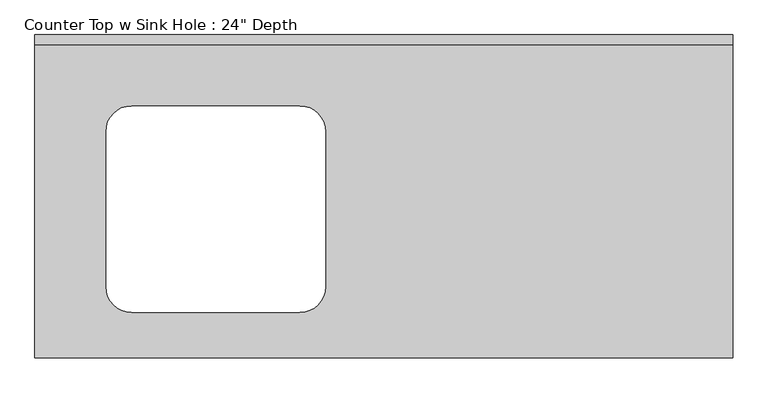
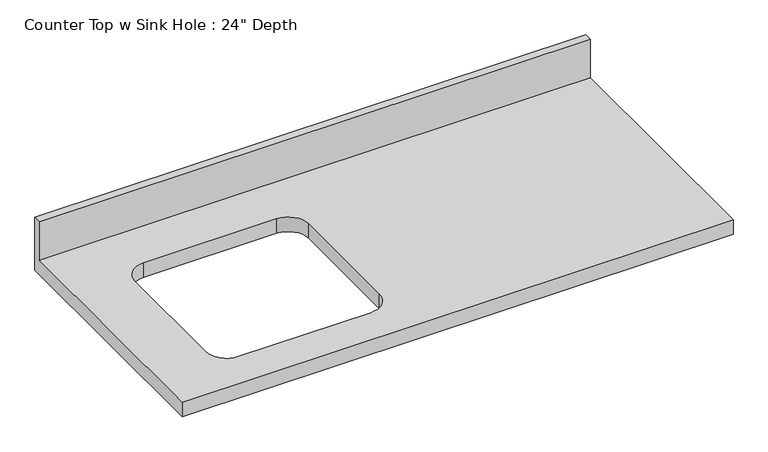
"""IFC4 building model written with IfcOpenShell, lengths in millimetres: furniture geometry."""

from ifc_helpers import new_model, si_unit, frame, origin, place, context, project, spatial, polyline, circle_curve, source, transform, mapped, element, save
from ifc_brep_helpers import plane_surface, revolved_surface, advanced_brep


def furniture_b3f308bd(model_context):
    return source(origin(), model_context, "Body", "AdvancedBrep", [
        advanced_brep(
        [(-1200.4622951, -635.0, 914.4), (171.1377049, -635.0, 914.4), (171.1377049, -19.05, 914.4), (-1200.4622951, -19.05, 914.4), (-1009.9622951, -139.7, 914.4), (-679.7622951, -139.7, 914.4), (-628.9622951, -190.5, 914.4), (-628.9622951, -495.3, 914.4), (-679.7622951, -546.1, 914.4), (-1009.9622951, -546.1, 914.4), (-1060.7622951, -495.3, 914.4), (-1060.7622951, -190.5, 914.4), (171.1377049, 0.0, 876.3), (171.1377049, -635.0, 876.3), (-1200.4622951, -635.0, 876.3), (-1200.4622951, 0.0, 876.3), (-679.7622951, -139.7, 876.3), (-1009.9622951, -139.7, 876.3), (-1060.7622951, -190.5, 876.3), (-1060.7622951, -495.3, 876.3), (-1009.9622951, -546.1, 876.3), (-679.7622951, -546.1, 876.3), (-628.9622951, -495.3, 876.3), (-628.9622951, -190.5, 876.3), (-1200.4622951, 0.0, 1016.0), (171.1377049, 0.0, 1016.0), (-1200.4622951, -19.05, 1016.0), (171.1377049, -19.05, 1016.0)],
        [
            (0, 1),
            (1, 2),
            (2, 3),
            (3, 0),
            (4, 5),
            (5, 6, circle_curve(frame((-679.7622951, -190.5, 914.4), z_axis=(0.0, 0.0, -1.0), x_axis=(1.0, 0.0, 0.0)), 50.8)),
            (6, 7),
            (7, 8, circle_curve(frame((-679.7622951, -495.3, 914.4), z_axis=(0.0, 0.0, -1.0), x_axis=(1.0, 0.0, 0.0)), 50.8)),
            (8, 9),
            (9, 10, circle_curve(frame((-1009.9622951, -495.3, 914.4), z_axis=(0.0, 0.0, -1.0), x_axis=(1.0, 0.0, 0.0)), 50.8)),
            (10, 11),
            (11, 4, circle_curve(frame((-1009.9622951, -190.5, 914.4), z_axis=(0.0, 0.0, -1.0), x_axis=(1.0, 0.0, 0.0)), 50.8)),
            (12, 13),
            (13, 14),
            (14, 15),
            (15, 12),
            (16, 17),
            (17, 18, circle_curve(frame((-1009.9622951, -190.5, 876.3), z_axis=(0.0, 0.0, 1.0), x_axis=(1.0, 0.0, 0.0)), 50.8)),
            (18, 19),
            (19, 20, circle_curve(frame((-1009.9622951, -495.3, 876.3), z_axis=(0.0, 0.0, 1.0), x_axis=(1.0, 0.0, 0.0)), 50.8)),
            (20, 21),
            (21, 22, circle_curve(frame((-679.7622951, -495.3, 876.3), z_axis=(0.0, 0.0, 1.0), x_axis=(1.0, 0.0, 0.0)), 50.8)),
            (22, 23),
            (23, 16, circle_curve(frame((-679.7622951, -190.5, 876.3), z_axis=(0.0, 0.0, 1.0), x_axis=(1.0, 0.0, 0.0)), 50.8)),
            (15, 24),
            (24, 25),
            (25, 12),
            (14, 0),
            (3, 26),
            (26, 24),
            (13, 1),
            (25, 27),
            (27, 2),
            (4, 17),
            (16, 5),
            (11, 18),
            (10, 19),
            (9, 20),
            (8, 21),
            (7, 22),
            (6, 23),
            (26, 27),
        ],
        [
            plane_surface(frame((-1200.4622951, 0.0, 914.4), z_axis=(0.0, 0.0, 1.0), x_axis=(-1.0, 0.0, 0.0))),
            plane_surface(frame((-1200.4622951, 0.0, 876.3), z_axis=(0.0, 0.0, -1.0), x_axis=(1.0, 0.0, 0.0))),
            plane_surface(frame((171.1377049, 0.0, 914.4), z_axis=(0.0, 1.0, 0.0), x_axis=(0.0, 0.0, -1.0))),
            plane_surface(frame((-1200.4622951, 0.0, 914.4), z_axis=(-1.0, 0.0, 0.0), x_axis=(0.0, 0.0, -1.0))),
            plane_surface(frame((-1200.4622951, -635.0, 914.4), z_axis=(0.0, -1.0, 0.0), x_axis=(0.0, 0.0, -1.0))),
            plane_surface(frame((171.1377049, -635.0, 914.4), z_axis=(1.0, 0.0, 0.0), x_axis=(0.0, 0.0, -1.0))),
            plane_surface(frame((-679.7622951, -139.7, 914.4), z_axis=(0.0, -1.0, 0.0), x_axis=(0.0, 0.0, -1.0))),
            revolved_surface(polyline([(-959.1622951, -190.5, 914.4), (-959.1622951, -190.5, 876.3)]), (-1009.9622951, -190.5, 876.3), (0.0, 0.0, 1.0)),
            plane_surface(frame((-1060.7622951, -190.5, 914.4), z_axis=(1.0, 0.0, 0.0), x_axis=(0.0, 0.0, -1.0))),
            revolved_surface(polyline([(-959.1622951, -495.3, 914.4), (-959.1622951, -495.3, 876.3)]), (-1009.9622951, -495.3, 876.3), (0.0, 0.0, 1.0)),
            plane_surface(frame((-1009.9622951, -546.1, 914.4), z_axis=(0.0, 1.0, 0.0), x_axis=(0.0, 0.0, -1.0))),
            revolved_surface(polyline([(-628.9622951, -495.3, 914.4), (-628.9622951, -495.3, 876.3)]), (-679.7622951, -495.3, 876.3), (0.0, 0.0, 1.0)),
            plane_surface(frame((-628.9622951, -495.3, 914.4), z_axis=(-1.0, 0.0, 0.0), x_axis=(0.0, 0.0, -1.0))),
            revolved_surface(polyline([(-628.9622951, -190.5, 914.4), (-628.9622951, -190.5, 876.3)]), (-679.7622951, -190.5, 876.3), (0.0, 0.0, 1.0)),
            plane_surface(frame((-1200.4622951, 0.0, 1016.0), z_axis=(0.0, 0.0, 1.0), x_axis=(0.0, -1.0, 0.0))),
            plane_surface(frame((-1200.4622951, -19.05, 1016.0), z_axis=(0.0, -1.0, 0.0), x_axis=(0.0, 0.0, -1.0))),
        ],
        [
            (0, [[1, 2, 3, 4], [5, 6, 7, 8, 9, 10, 11, 12]]),
            (1, [[13, 14, 15, 16], [17, 18, 19, 20, 21, 22, 23, 24]]),
            (2, [[-16, 25, 26, 27]]),
            (3, [[-15, 28, -4, 29, 30, -25]]),
            (4, [[-1, -28, -14, 31]]),
            (5, [[-13, -27, 32, 33, -2, -31]]),
            (6, [[34, -17, 35, -5]]),
            (7, [[-34, -12, 36, -18]]),
            (8, [[-36, -11, 37, -19]]),
            (9, [[-37, -10, 38, -20]]),
            (10, [[-38, -9, 39, -21]]),
            (11, [[-39, -8, 40, -22]]),
            (12, [[-40, -7, 41, -23]]),
            (13, [[-35, -24, -41, -6]]),
            (14, [[-30, 42, -32, -26]]),
            (15, [[-42, -29, -3, -33]]),
        ],
    ),
    ])


if __name__ == "__main__":
    model = new_model("IFC4")
    model_context = context("Model", 3, world=origin())
    ifc_project = project(units=[si_unit("LENGTHUNIT", "METRE", prefix="MILLI")], contexts=[model_context])
    site = spatial("IfcSite", under=ifc_project)
    building = spatial("IfcBuilding", under=site)
    placement = place(None, origin())
    furniture_shape = furniture_b3f308bd(model_context)
    element("IfcFurniture", 1, ObjectType="Counter Top w Sink Hole : 24\" Depth", at=placement, inside=building, context=model_context, shape_type="MappedRepresentation", body=[
        mapped(furniture_shape, transform((0.0, 0.0, 0.0), x_axis=(1.0, 0.0, 0.0), y_axis=(0.0, 1.0, 0.0), z_axis=(0.0, 0.0, 1.0))),
    ])
    save(model, "model.ifc")

# Revit data of these elements
# Type "Counter Top w Sink Hole : 24\" Depth"
#   Assembly Code = "C1030400"
#   Counter Thickness = 0' - 1 1/2"
#   Depth = 2' - 1"
#   Height = 3' - 0"
#   Length [instance default] = 8' - 0"
#   Sink Location [instance default] = 2' - 0"
#   Sink Location To Wall [instance default] = 0' - 6"
#   Sink Opening Depth [instance default] = 1' - 3"
#   Sink Opening Width [instance default] = 2' - 3"
#   Counter Top Material = none
#   Default Elevation = 0
# Element 1 (IfcFurniture, "Counter Top w Sink Hole : 24\" Depth")
#   Length = 4' - 6"
#   Sink Location = 1' - 2"
#   Sink Opening Width = 1' - 4"
#   Materials on its faces: "Counter Top"
# Materials
#   "Counter Top": class "Wood", colour RGB 226 177 128, transparency 0
